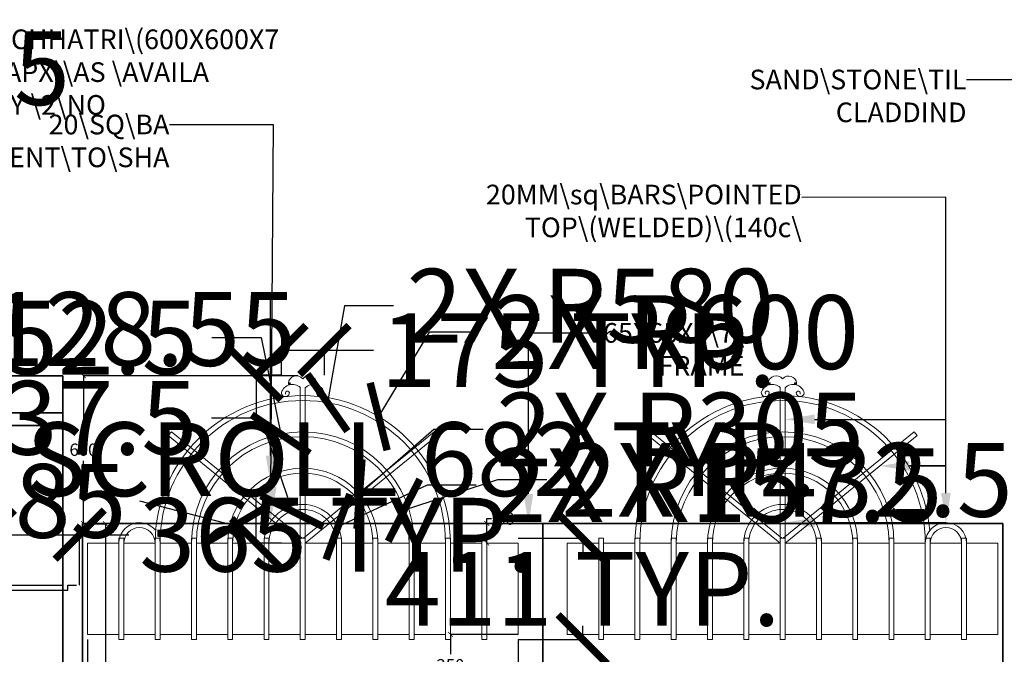
# Model space of a CAD drawing. Units: millimetres. Extents: x 16635 to 28332, y 17519 to 22633.
# Tile 3 of 4: x 20029 to 24031, y 20054 to 22633. Entities that reach past the tile are written whole.
import ezdxf
from ezdxf import colors
from ezdxf.entities.mleader import LeaderData, LeaderLine
from ezdxf.math import Vec2, Vec3

# ---------------------------------------------------------------- set-up
doc = ezdxf.new("R2010")
doc.units = ezdxf.units.MM
doc.header["$MEASUREMENT"] = 0
for name, color, linetype, lineweight in [('A-ANNO-DIMS', 2, 'Continuous', 18), ('A-ANNO-TEXT', 7, 'Continuous', 18), ('A-GATE', 3, 'Continuous', 35), ('A-GATE-GRIL', 4, 'Continuous', 18), ('A-GATE-HRDW', 3, 'Continuous', 25), ('A-WALL', 7, 'Continuous', 35)]:
    doc.layers.add(name, color=color, linetype=linetype, lineweight=lineweight)
doc.styles.get("Standard").update_dxf_attribs({"font": 'arial.ttf'})
doc.dimstyles.get("Standard").update_dxf_attribs({"dimtxt": 300, "dimasz": 200, "dimexe": 0.18, "dimexo": 0.0625, "dimgap": 0.09, "dimtad": 0, "dimtih": 1, "dimtoh": 1, "dimdec": 0, "dimzin": 0, "dimdsep": 46, "dimtxsty": 'Standard', "dimblk": 'ARCHTICK', "dimcen": 0.09, "dimadec": 0, "dimazin": 0, "dimtfac": 1, "dimtdec": 0, "dimtofl": 0, "dimtmove": 0, "dimatfit": 3, "dimfxl": 1, "dimtolj": 1, "dimtzin": 0, "dimarcsym": 0})

# ---------------------------------------------------------------- blocks, each defined once
blk = doc.blocks.new('_ArchTick')
at = {"color": 0, "linetype": 'ByBlock', "const_width": 0.15}
blk.add_lwpolyline([(-0.5, -0.5), (0.5, 0.5)], dxfattribs=at)
blk = doc.blocks.new('*D8')
at = {"layer": 'A-ANNO-DIMS', "color": 0, "lineweight": -2, "transparency": 16777216}
for p, q in [((21159.1, 21185.3), (20288.1, 21185.3)), ((20288.3, 21185.3), (20288.3, 20930.9)), ((20288.3, 20585.3), (20288.3, 20839.8)), ((20284.8, 20585.3), (20288.5, 20585.3))]:
    blk.add_line(p, q, dxfattribs=at)
at = {"layer": 'Defpoints', "color": 0, "transparency": 16777216}
for p in [(20288.3, 21185.3), (21159.1, 21185.3), (20284.8, 20585.3)]:
    blk.add_point(p, dxfattribs=at)
at = {"layer": 'A-ANNO-DIMS', "color": 0, "lineweight": -2, "transparency": 16777216, "xscale": 20, "yscale": 20, "zscale": 20}
for p, rotation in [((20288.3, 21185.3), 90), ((20288.3, 20585.3), 270)]:
    blk.add_blockref('_ArchTick', p, dxfattribs=dict(at, rotation=rotation))
at = {"layer": 'A-ANNO-DIMS', "color": 0, "transparency": 16777216, "insert": (20288.3, 20885.3), "char_height": 50, "attachment_point": 5}
blk.add_mtext('\\A1;600', dxfattribs=at)
blk = doc.blocks.new('*D13')
at = {"layer": 'A-ANNO-DIMS', "color": 0, "lineweight": -2, "transparency": 16777216}
for p, q in [((20284.8, 20584.3), (20377.6, 20584.3)), ((20377.4, 20584.3), (20377.4, 19704.9)), ((20377.4, 18734.3), (20377.4, 19613.8)), ((20284.8, 18734.3), (20377.6, 18734.3))]:
    blk.add_line(p, q, dxfattribs=at)
at = {"layer": 'Defpoints', "color": 0, "transparency": 16777216}
for p in [(20284.8, 20584.3), (20284.8, 18734.3), (20377.4, 18734.3)]:
    blk.add_point(p, dxfattribs=at)
at = {"layer": 'A-ANNO-DIMS', "color": 0, "lineweight": -2, "transparency": 16777216, "xscale": 20, "yscale": 20, "zscale": 20}
for p, rotation in [((20377.4, 20584.3), 90), ((20377.4, 18734.3), 270)]:
    blk.add_blockref('_ArchTick', p, dxfattribs=dict(at, rotation=rotation))
at = {"layer": 'A-ANNO-DIMS', "color": 0, "transparency": 16777216, "insert": (20377.4, 19659.3), "char_height": 50, "attachment_point": 5}
blk.add_mtext('\\A1;1850', dxfattribs=at)
blk = doc.blocks.new('*D14')
at = {"layer": 'A-ANNO-DIMS', "color": 0, "lineweight": -2, "transparency": 16777216}
for p, q in [((22054.7, 20134.3), (21779.6, 20134.3)), ((21779.8, 20134.3), (21779.8, 20054.9)), ((21779.8, 19884.3), (21779.8, 19963.8)), ((22054.7, 19884.3), (21779.6, 19884.3))]:
    blk.add_line(p, q, dxfattribs=at)
at = {"layer": 'Defpoints', "color": 0, "transparency": 16777216}
for p in [(22054.8, 20134.3), (21779.8, 19884.3), (22054.8, 19884.3)]:
    blk.add_point(p, dxfattribs=at)
at = {"layer": 'A-ANNO-DIMS', "color": 0, "lineweight": -2, "transparency": 16777216, "xscale": 20, "yscale": 20, "zscale": 20}
for p, rotation in [((21779.8, 20134.3), 90), ((21779.8, 19884.3), 270)]:
    blk.add_blockref('_ArchTick', p, dxfattribs=dict(at, rotation=rotation))
at = {"layer": 'A-ANNO-DIMS', "color": 0, "transparency": 16777216, "insert": (21779.8, 20009.3), "char_height": 50, "attachment_point": 5}
blk.add_mtext('\\A1;250', dxfattribs=at)
blk = doc.blocks.new('*D15')
at = {"layer": 'A-ANNO-DIMS', "color": 0, "lineweight": -2, "transparency": 16777216}
for p, q in [((21927.3, 20585.3), (21927.3, 20605.3)), ((21927.3, 20605.3), (21947.3, 20605.3)), ((21927.3, 20585.3), (21927.5, 20585.3)), ((21927.3, 20505.3), (21927.3, 20585.3)), ((21927.3, 20505.3), (21927.5, 20505.3))]:
    blk.add_line(p, q, dxfattribs=at)
at = {"layer": 'Defpoints', "color": 0, "transparency": 16777216}
for p in [(21927.3, 20585.3), (21927.3, 20585.3), (21927.3, 20505.3)]:
    blk.add_point(p, dxfattribs=at)
at = {"layer": 'A-ANNO-DIMS', "color": 0, "lineweight": -2, "transparency": 16777216, "xscale": 20, "yscale": 20, "zscale": 20}
for p, rotation in [((21927.3, 20585.3), 90), ((21927.3, 20505.3), 270)]:
    blk.add_blockref('_ArchTick', p, dxfattribs=dict(at, rotation=rotation))
at = {"layer": 'A-ANNO-DIMS', "color": 0, "transparency": 16777216, "insert": (22003, 20605.3), "char_height": 50, "attachment_point": 5}
blk.add_mtext('\\A1;80', dxfattribs=at)
blk = doc.blocks.new('GATE-GRILLE-UPPER')
for p, q in [((127.5, 391), (127.5, 411)), ((127.5, 411), (147.5, 411)), ((147.5, 411), (147.5, 391)), ((275, 391), (275, 411)), ((275, 411), (295, 411)), ((295, 411), (295, 391)), ((422.5, 391), (422.5, 411)), ((422.5, 411), (442.5, 411)), ((442.5, 411), (442.5, 391)), ((570, 391), (570, 411)), ((570, 411), (590, 411)), ((590, 411), (590, 391)), ((717.5, 391), (717.5, 411)), ((717.5, 411), (737.5, 411)), ((737.5, 411), (737.5, 391)), ((865, 411), (885, 411)), ((1012.5, 391), (1012.5, 411)), ((1012.5, 411), (1032.5, 411)), ((1032.5, 411), (1032.5, 391)), ((1160, 391), (1160, 411)), ((1160, 411), (1180, 411)), ((1180, 411), (1180, 391)), ((1307.5, 391), (1307.5, 411)), ((1307.5, 411), (1327.5, 411)), ((1327.5, 411), (1327.5, 391)), ((1455, 391), (1455, 411)), ((1455, 411), (1475, 411)), ((1475, 411), (1475, 391)), ((1602.5, 391), (1602.5, 411)), ((1602.5, 411), (1622.5, 411)), ((1622.5, 411), (1622.5, 391)), ((0, 20), (0, 391)), ((0, 391), (127.5, 391)), ((127.5, 20), (127.5, 391)), ((127.5, 390.5), (127.5, 391)), ((147.5, 20), (147.5, 391)), ((147.5, 390.5), (147.5, 391)), ((147.5, 391), (275, 391)), ((275, 20), (275, 391)), ((275, 390.5), (275, 391)), ((295, 20), (295, 391)), ((295, 390.5), (295, 391)), ((295, 391), (422.5, 391)), ((422.5, 20), (422.5, 391)), ((422.5, 390.5), (422.5, 391)), ((442.5, 20), (442.5, 391)), ((442.5, 390.5), (442.5, 391)), ((442.5, 391), (570, 391)), ((570, 20), (570, 391)), ((570, 390.5), (570, 391)), ((590, 20), (590, 391)), ((590, 390.5), (590, 391)), ((590, 391), (717.5, 391)), ((717.5, 20), (717.5, 391)), ((717.5, 390.5), (717.5, 391)), ((737.5, 20), (737.5, 391)), ((737.5, 390.5), (737.5, 391)), ((737.5, 391), (865, 391)), ((865, 20), (865, 391)), ((865, 390.5), (865, 391)), ((885, 20), (885, 391)), ((885, 390.5), (885, 391)), ((885, 391), (1012.5, 391)), ((1012.5, 20), (1012.5, 391)), ((1012.5, 390.5), (1012.5, 391)), ((1032.5, 20), (1032.5, 391)), ((1032.5, 390.5), (1032.5, 391)), ((1032.5, 391), (1160, 391)), ((1160, 20), (1160, 391)), ((1160, 390.5), (1160, 391)), ((1180, 20), (1180, 391)), ((1180, 390.5), (1180, 391)), ((1180, 391), (1307.5, 391)), ((1307.5, 20), (1307.5, 391)), ((1307.5, 390.5), (1307.5, 391)), ((1327.5, 20), (1327.5, 391)), ((1327.5, 390.5), (1327.5, 391)), ((1327.5, 391), (1455, 391)), ((1455, 20), (1455, 391)), ((1455, 390.5), (1455, 391)), ((1475, 20), (1475, 391)), ((1475, 390.5), (1475, 391)), ((1475, 391), (1602.5, 391)), ((1602.5, 20), (1602.5, 391)), ((1602.5, 390.5), (1602.5, 391)), ((1622.5, 20), (1622.5, 391)), ((1622.5, 390.5), (1622.5, 391)), ((1622.5, 391), (1750, 391)), ((1750, 20), (1750, 391)), ((1750, 390.5), (1750, 391)), ((0, 20), (127.5, 20)), ((127.5, 20), (127.5, 0)), ((147.5, 0), (147.5, 20)), ((147.5, 20), (275, 20)), ((275, 20), (275, 0)), ((295, 0), (295, 20)), ((295, 20), (422.5, 20)), ((422.5, 20), (422.5, 0)), ((442.5, 0), (442.5, 20)), ((442.5, 20), (570, 20)), ((570, 20), (570, 0)), ((590, 0), (590, 20)), ((590, 20), (717.5, 20)), ((717.5, 20), (717.5, 0)), ((737.5, 0), (737.5, 20)), ((737.5, 20), (865, 20)), ((865, 20), (865, 0)), ((885, 0), (885, 20)), ((885, 20), (1012.5, 20)), ((1012.5, 20), (1012.5, 0)), ((1032.5, 0), (1032.5, 20)), ((1032.5, 20), (1160, 20)), ((1160, 20), (1160, 0)), ((1180, 0), (1180, 20)), ((1180, 20), (1307.5, 20)), ((1307.5, 20), (1307.5, 0)), ((1327.5, 0), (1327.5, 20)), ((1327.5, 20), (1455, 20)), ((1455, 20), (1455, 0)), ((1475, 0), (1475, 20)), ((1475, 20), (1602.5, 20)), ((1602.5, 20), (1602.5, 0)), ((1622.5, 0), (1622.5, 20)), ((1622.5, 20), (1750, 20)), ((127.5, 0), (147.5, 0)), ((275, 0), (295, 0)), ((422.5, 0), (442.5, 0)), ((570, 0), (590, 0)), ((717.5, 0), (737.5, 0)), ((865, 0), (885, 0)), ((1012.5, 0), (1032.5, 0)), ((1160, 0), (1180, 0)), ((1307.5, 0), (1327.5, 0)), ((1455, 0), (1475, 0)), ((1602.5, 0), (1622.5, 0))]:
    blk.add_line(p, q)
blk = doc.blocks.new('GATE-CREST-SCROLL')
for p, q in [((76.7, 0), (76.7, 632.5)), ((96.7, 632.1), (96.7, 0))]:
    blk.add_line(p, q)
for centre, radius, start, end in [((44.6, 598.6), 46.7, 46.5386, 162.6285), ((61.2, 646.7), 33.3, 40.0087, 174.5179), ((32.3, 649.8), 4.3, 170.4451, 358.3477), ((34.4, 649.3), 2.21, 12.093, 205.0593), ((111.4, 647.2), 32.3, 5.8157, 139.8182), ((129.3, 598.6), 46.7, 15.1459, 134.1823), ((137.2, 649.2), 2.21, 334.9407, 167.907), ((139.3, 649.8), 4.3, 181.6523, 9.5549), ((16.2, 611.9), 16.2, 177.7213, 358.3477), ((24.2, 609.7), 8.33, 12.093, 205.0593), ((150.2, 609.7), 8.33, 334.9407, 167.907), ((158.2, 611.9), 16.2, 181.6523, 356.1099)]:
    blk.add_arc(centre, radius, start, end)
blk = doc.blocks.new('GATE-JAMB-ANCHOR-SET')
for p, q in [((0.2, 1370), (297.2, 1370)), ((317.2, 1350), (317.2, 1370)), ((317.2, 1370), (351.9, 1370)), ((0.2, 1350), (297.2, 1350)), ((297.2, 1350), (317.2, 1350)), ((0, 694.8), (297, 694.8)), ((317, 674.8), (317, 694.8)), ((317, 694.8), (365.3, 694.8)), ((0, 674.8), (297, 674.8)), ((297, 674.8), (317, 674.8)), ((0.2, 20), (297.2, 20)), ((317.2, 0), (317.2, 20)), ((317.2, 20), (360.9, 20)), ((0.2, 0), (297.2, 0)), ((297.2, 0), (317.2, 0))]:
    blk.add_line(p, q)
blk = doc.blocks.new('*D45')
at = {"layer": 'A-ANNO-DIMS', "color": 0, "lineweight": -2, "transparency": 16777216}
for p, q in [((20304.8, 20114.3), (20304.8, 19851.7)), ((22054.8, 20114.3), (22054.8, 19851.7)), ((20304.8, 19851.8), (22054.8, 19851.8)), ((22054.8, 19851.8), (22254.8, 19851.8))]:
    blk.add_line(p, q, dxfattribs=at)
at = {"layer": 'Defpoints', "color": 0, "transparency": 16777216}
for p in [(20304.8, 20114.3), (22054.8, 20114.3), (22054.8, 19851.8)]:
    blk.add_point(p, dxfattribs=at)
at = {"layer": 'A-ANNO-DIMS', "color": 0, "lineweight": -2, "transparency": 16777216, "xscale": 200, "yscale": 200, "zscale": 200, "rotation": 180}
blk.add_blockref('_ArchTick', (20304.8, 19851.8), dxfattribs=at)
at = {"layer": 'A-ANNO-DIMS', "color": 0, "lineweight": -2, "transparency": 16777216, "xscale": 200, "yscale": 200, "zscale": 200}
blk.add_blockref('_ArchTick', (22054.8, 19851.8), dxfattribs=at)
at = {"layer": 'A-ANNO-DIMS', "color": 0, "transparency": 16777216, "insert": (24794.1, 19851.8), "char_height": 300, "attachment_point": 5}
blk.add_mtext('\\A1;UPPER GRILLE 1750 TYP.', dxfattribs=at)
blk = doc.blocks.new('*D46')
at = {"layer": 'A-ANNO-DIMS', "color": 0, "lineweight": -2, "transparency": 16777216}
for p, q in [((22054.8, 20525.3), (22317.5, 20525.3)), ((22317.3, 20525.3), (22317.3, 20470.7)), ((22317.3, 20114.3), (22317.3, 20169)), ((22054.8, 20114.3), (22317.5, 20114.3))]:
    blk.add_line(p, q, dxfattribs=at)
at = {"layer": 'Defpoints', "color": 0, "transparency": 16777216}
for p in [(22054.8, 20525.3), (22317.3, 20525.3), (22054.8, 20114.3)]:
    blk.add_point(p, dxfattribs=at)
at = {"layer": 'A-ANNO-DIMS', "color": 0, "lineweight": -2, "transparency": 16777216, "xscale": 200, "yscale": 200, "zscale": 200}
for p, rotation in [((22317.3, 20525.3), 90), ((22317.3, 20114.3), 270)]:
    blk.add_blockref('_ArchTick', p, dxfattribs=dict(at, rotation=rotation))
at = {"layer": 'A-ANNO-DIMS', "color": 0, "transparency": 16777216, "insert": (22317.3, 20319.8), "char_height": 300, "attachment_point": 5}
blk.add_mtext('\\A1;411 TYP.', dxfattribs=at)
blk = doc.blocks.new('*D47')
at = {"layer": 'A-ANNO-DIMS', "color": 0, "lineweight": -2, "transparency": 16777216}
for p, q in [((21092.8, 21187.8), (20990.3, 21187.8)), ((20990.5, 21187.8), (20990.5, 21001.9)), ((20990.5, 20505.3), (20990.5, 20691.3)), ((21092.8, 20505.3), (20990.3, 20505.3))]:
    blk.add_line(p, q, dxfattribs=at)
at = {"layer": 'Defpoints', "color": 0, "transparency": 16777216}
for p in [(20990.5, 21187.8), (21092.8, 21187.8), (21092.8, 20505.3)]:
    blk.add_point(p, dxfattribs=at)
at = {"layer": 'A-ANNO-DIMS', "color": 0, "lineweight": -2, "transparency": 16777216, "xscale": 200, "yscale": 200, "zscale": 200}
for p, rotation in [((20990.5, 21187.8), 90), ((20990.5, 20505.3), 270)]:
    blk.add_blockref('_ArchTick', p, dxfattribs=dict(at, rotation=rotation))
at = {"layer": 'A-ANNO-DIMS', "color": 0, "transparency": 16777216, "insert": (20990.5, 20846.6), "char_height": 300, "attachment_point": 5}
blk.add_mtext('\\A1;CREST SCROLL 682 TYP.', dxfattribs=at)
blk = doc.blocks.new('*D48')
at = {"layer": 'A-ANNO-DIMS', "color": 0, "lineweight": -2, "transparency": 16777216}
for p, q in [((21092.8, 21187.9), (21092.8, 21290.4)), ((21092.8, 21290.2), (21267.4, 21290.2)), ((21267.4, 21187.9), (21267.4, 21290.4)), ((21267.4, 21290.2), (21467.4, 21290.2))]:
    blk.add_line(p, q, dxfattribs=at)
at = {"layer": 'Defpoints', "color": 0, "transparency": 16777216}
for p in [(21267.4, 21290.2), (21092.8, 21187.8), (21267.4, 21187.8)]:
    blk.add_point(p, dxfattribs=at)
at = {"layer": 'A-ANNO-DIMS', "color": 0, "lineweight": -2, "transparency": 16777216, "xscale": 200, "yscale": 200, "zscale": 200, "rotation": 180}
blk.add_blockref('_ArchTick', (21092.8, 21290.2), dxfattribs=at)
at = {"layer": 'A-ANNO-DIMS', "color": 0, "lineweight": -2, "transparency": 16777216, "xscale": 200, "yscale": 200, "zscale": 200}
blk.add_blockref('_ArchTick', (21267.4, 21290.2), dxfattribs=at)
at = {"layer": 'A-ANNO-DIMS', "color": 0, "transparency": 16777216, "insert": (22300.1, 21290.2), "char_height": 300, "attachment_point": 5}
blk.add_mtext('\\A1;175 TYP.', dxfattribs=at)
blk = doc.blocks.new('*D49')
at = {"layer": 'A-ANNO-DIMS', "color": 0, "lineweight": -2, "transparency": 16777216}
for p, q in [((19907.5, 20334.3), (19701.9, 20334.3)), ((19702.1, 20334.3), (19702.1, 19804.8)), ((19702.1, 18964.3), (19702.1, 19493.9)), ((19907.5, 18964.3), (19701.9, 18964.3))]:
    blk.add_line(p, q, dxfattribs=at)
at = {"layer": 'Defpoints', "color": 0, "transparency": 16777216}
for p in [(19702.1, 20334.3), (19907.6, 20334.3), (19907.6, 18964.3)]:
    blk.add_point(p, dxfattribs=at)
at = {"layer": 'A-ANNO-DIMS', "color": 0, "lineweight": -2, "transparency": 16777216, "xscale": 200, "yscale": 200, "zscale": 200}
for p, rotation in [((19702.1, 20334.3), 90), ((19702.1, 18964.3), 270)]:
    blk.add_blockref('_ArchTick', p, dxfattribs=dict(at, rotation=rotation))
at = {"layer": 'A-ANNO-DIMS', "color": 0, "transparency": 16777216, "insert": (19702.1, 19649.3), "char_height": 300, "attachment_point": 5}
blk.add_mtext('\\A1;JAMB ANCHORS 1370 TYP.', dxfattribs=at)
blk = doc.blocks.new('*D50')
at = {"layer": 'A-ANNO-DIMS', "color": 0, "lineweight": -2, "transparency": 16777216}
for p, q in [((19907.6, 20334.4), (19907.6, 20540)), ((19907.6, 20539.8), (20272.8, 20539.8)), ((20272.8, 20334.4), (20272.8, 20540)), ((20272.8, 20539.8), (20472.8, 20539.8))]:
    blk.add_line(p, q, dxfattribs=at)
at = {"layer": 'Defpoints', "color": 0, "transparency": 16777216}
for p in [(20272.8, 20539.8), (19907.6, 20334.3), (20272.8, 20334.3)]:
    blk.add_point(p, dxfattribs=at)
at = {"layer": 'A-ANNO-DIMS', "color": 0, "lineweight": -2, "transparency": 16777216, "xscale": 200, "yscale": 200, "zscale": 200, "rotation": 180}
blk.add_blockref('_ArchTick', (19907.6, 20539.8), dxfattribs=at)
at = {"layer": 'A-ANNO-DIMS', "color": 0, "lineweight": -2, "transparency": 16777216, "xscale": 200, "yscale": 200, "zscale": 200}
blk.add_blockref('_ArchTick', (20272.8, 20539.8), dxfattribs=at)
at = {"layer": 'A-ANNO-DIMS', "color": 0, "transparency": 16777216, "insert": (21319.5, 20539.8), "char_height": 300, "attachment_point": 5}
blk.add_mtext('\\A1;365 TYP.', dxfattribs=at)
blk = doc.blocks.new('*D59')
at = {"layer": 'A-ANNO-DIMS', "color": 0, "lineweight": -2, "transparency": 16777216}
for p, q in [((18754.8, 20334.4), (18754.8, 22436.4)), ((18754.8, 22436.2), (19012.3, 22436.2)), ((19012.3, 21184.4), (19012.3, 22436.4)), ((19012.3, 22436.2), (19212.3, 22436.2))]:
    blk.add_line(p, q, dxfattribs=at)
at = {"layer": 'Defpoints', "color": 0, "transparency": 16777216}
for p in [(19012.3, 22436.2), (19012.3, 21184.3), (18754.8, 20334.3)]:
    blk.add_point(p, dxfattribs=at)
at = {"layer": 'A-ANNO-DIMS', "color": 0, "lineweight": -2, "transparency": 16777216, "xscale": 200, "yscale": 200, "zscale": 200, "rotation": 180}
blk.add_blockref('_ArchTick', (18754.8, 22436.2), dxfattribs=at)
at = {"layer": 'A-ANNO-DIMS', "color": 0, "lineweight": -2, "transparency": 16777216, "xscale": 200, "yscale": 200, "zscale": 200}
blk.add_blockref('_ArchTick', (19012.3, 22436.2), dxfattribs=at)
at = {"layer": 'A-ANNO-DIMS', "color": 0, "transparency": 16777216, "insert": (19722.2, 22436.2), "char_height": 300, "attachment_point": 5}
blk.add_mtext('\\A1;257.5', dxfattribs=at)
blk = doc.blocks.new('*D66')
at = {"layer": 'A-ANNO-DIMS', "color": 0, "lineweight": -2, "transparency": 16777216}
for p, q in [((19003.3, 21688.7), (19003.5, 21688.7)), ((19003.4, 21688.6), (19003.4, 21688.7)), ((19429.5, 21375.9), (19107.1, 21612.6)), ((19629.5, 21375.9), (19429.5, 21375.9))]:
    blk.add_line(p, q, dxfattribs=at)
at = {"layer": 'Defpoints', "color": 0, "transparency": 16777216}
for p in [(19003.4, 21688.7), (19107.1, 21612.6)]:
    blk.add_point(p, dxfattribs=at)
at = {"layer": 'A-ANNO-DIMS', "color": 0, "lineweight": -2, "transparency": 16777216, "xscale": 200, "yscale": 200, "zscale": 200, "rotation": 143.726603085954}
blk.add_blockref('_ArchTick', (19107.1, 21612.6), dxfattribs=at)
at = {"layer": 'A-ANNO-DIMS', "color": 0, "transparency": 16777216, "insert": (20397, 21375.9), "char_height": 300, "attachment_point": 5}
blk.add_mtext('\\A1;R128.55', dxfattribs=at)
blk = doc.blocks.new('*D67')
at = {"layer": 'A-ANNO-DIMS', "color": 0, "lineweight": -2, "transparency": 16777216}
for p, q in [((21693.6, 21363.3), (21488.1, 21020.1)), ((21893.6, 21363.3), (21693.6, 21363.3)), ((21179.7, 20505.3), (21179.9, 20505.3)), ((21179.8, 20505.3), (21179.8, 20505.4))]:
    blk.add_line(p, q, dxfattribs=at)
at = {"layer": 'Defpoints', "color": 0, "transparency": 16777216}
for p in [(21488.1, 21020.1), (21179.8, 20505.3)]:
    blk.add_point(p, dxfattribs=at)
at = {"layer": 'A-ANNO-DIMS', "color": 0, "lineweight": -2, "transparency": 16777216, "xscale": 200, "yscale": 200, "zscale": 200, "rotation": 239.0822028428942}
blk.add_blockref('_ArchTick', (21488.1, 21020.1), dxfattribs=at)
at = {"layer": 'A-ANNO-DIMS', "color": 0, "transparency": 16777216, "insert": (22693, 21363.3), "char_height": 300, "attachment_point": 5}
blk.add_mtext('\\A1;2X R600', dxfattribs=at)
blk = doc.blocks.new('*D68')
at = {"layer": 'A-ANNO-DIMS', "color": 0, "lineweight": -2, "transparency": 16777216}
for p, q in [((21349, 21470.6), (21279.9, 21076.6)), ((21549, 21470.6), (21349, 21470.6)), ((21179.7, 20505.3), (21179.9, 20505.3)), ((21179.8, 20505.3), (21179.8, 20505.4))]:
    blk.add_line(p, q, dxfattribs=at)
at = {"layer": 'Defpoints', "color": 0, "transparency": 16777216}
for p in [(21279.9, 21076.6), (21179.8, 20505.3)]:
    blk.add_point(p, dxfattribs=at)
at = {"layer": 'A-ANNO-DIMS', "color": 0, "lineweight": -2, "transparency": 16777216, "xscale": 200, "yscale": 200, "zscale": 200, "rotation": 260.0552103335245}
blk.add_blockref('_ArchTick', (21279.9, 21076.6), dxfattribs=at)
at = {"layer": 'A-ANNO-DIMS', "color": 0, "transparency": 16777216, "insert": (22348.4, 21470.6), "char_height": 300, "attachment_point": 5}
blk.add_mtext('\\A1;2X R580', dxfattribs=at)
blk = doc.blocks.new('*D69')
at = {"layer": 'A-ANNO-DIMS', "color": 0, "lineweight": -2, "transparency": 16777216}
for p, q in [((20810.7, 21340.9), (21010.7, 21340.9)), ((21010.7, 21340.9), (21090, 20948.9)), ((21179.7, 20505.3), (21179.9, 20505.3)), ((21179.8, 20505.3), (21179.8, 20505.4))]:
    blk.add_line(p, q, dxfattribs=at)
at = {"layer": 'Defpoints', "color": 0, "transparency": 16777216}
for p in [(21090, 20948.9), (21179.8, 20505.3)]:
    blk.add_point(p, dxfattribs=at)
at = {"layer": 'A-ANNO-DIMS', "color": 0, "lineweight": -2, "transparency": 16777216, "xscale": 200, "yscale": 200, "zscale": 200, "rotation": 281.4390211623567}
blk.add_blockref('_ArchTick', (21090, 20948.9), dxfattribs=at)
at = {"layer": 'A-ANNO-DIMS', "color": 0, "transparency": 16777216, "insert": (19834.9, 21340.9), "char_height": 300, "attachment_point": 5}
blk.add_mtext('\\A1;2X R452.5', dxfattribs=at)
blk = doc.blocks.new('*D70')
at = {"layer": 'A-ANNO-DIMS', "color": 0, "lineweight": -2, "transparency": 16777216}
for p, q in [((21971.5, 20762.6), (21591.1, 20639)), ((22171.5, 20762.6), (21971.5, 20762.6)), ((21179.7, 20505.3), (21179.9, 20505.3)), ((21179.8, 20505.3), (21179.8, 20505.4))]:
    blk.add_line(p, q, dxfattribs=at)
at = {"layer": 'Defpoints', "color": 0, "transparency": 16777216}
for p in [(21591.1, 20639), (21179.8, 20505.3)]:
    blk.add_point(p, dxfattribs=at)
at = {"layer": 'A-ANNO-DIMS', "color": 0, "lineweight": -2, "transparency": 16777216, "xscale": 200, "yscale": 200, "zscale": 200, "rotation": 198.0002935108227}
blk.add_blockref('_ArchTick', (21591.1, 20639), dxfattribs=at)
at = {"layer": 'A-ANNO-DIMS', "color": 0, "transparency": 16777216, "insert": (23147.3, 20762.6), "char_height": 300, "attachment_point": 5}
blk.add_mtext('\\A1;2X R432.5', dxfattribs=at)
blk = doc.blocks.new('*D71')
at = {"layer": 'A-ANNO-DIMS', "color": 0, "lineweight": -2, "transparency": 16777216}
for p, q in [((21712.4, 20967.2), (21410.2, 20705.2)), ((21912.4, 20967.2), (21712.4, 20967.2)), ((21179.7, 20505.3), (21179.9, 20505.3)), ((21179.8, 20505.3), (21179.8, 20505.4))]:
    blk.add_line(p, q, dxfattribs=at)
at = {"layer": 'Defpoints', "color": 0, "transparency": 16777216}
for p in [(21410.2, 20705.2), (21179.8, 20505.3)]:
    blk.add_point(p, dxfattribs=at)
at = {"layer": 'A-ANNO-DIMS', "color": 0, "lineweight": -2, "transparency": 16777216, "xscale": 200, "yscale": 200, "zscale": 200, "rotation": 220.9312972223516}
blk.add_blockref('_ArchTick', (21410.2, 20705.2), dxfattribs=at)
at = {"layer": 'A-ANNO-DIMS', "color": 0, "transparency": 16777216, "insert": (22713.4, 20967.2), "char_height": 300, "attachment_point": 5}
blk.add_mtext('\\A1;2X R305', dxfattribs=at)
blk = doc.blocks.new('*D72')
at = {"layer": 'A-ANNO-DIMS', "color": 0, "lineweight": -2, "transparency": 16777216}
for p, q in [((20516.7, 20677.3), (20903.9, 20576.9)), ((21179.7, 20505.3), (21179.9, 20505.3)), ((21179.8, 20505.3), (21179.8, 20505.4))]:
    blk.add_line(p, q, dxfattribs=at)
at = {"layer": 'Defpoints', "color": 0, "transparency": 16777216}
for p in [(20903.9, 20576.9), (21179.8, 20505.3)]:
    blk.add_point(p, dxfattribs=at)
at = {"layer": 'A-ANNO-DIMS', "color": 0, "lineweight": -2, "transparency": 16777216, "xscale": 200, "yscale": 200, "zscale": 200, "rotation": 345.4648454983082}
blk.add_blockref('_ArchTick', (20903.9, 20576.9), dxfattribs=at)
at = {"layer": 'A-ANNO-DIMS', "color": 0, "transparency": 16777216, "insert": (19715.6, 20677.3), "char_height": 300, "attachment_point": 5}
blk.add_mtext('\\A1;2X R285', dxfattribs=at)
blk = doc.blocks.new('*D73')
at = {"layer": 'A-ANNO-DIMS', "color": 0, "lineweight": -2, "transparency": 16777216}
for p, q in [((21685, 20740.9), (21322.5, 20571.9)), ((21885, 20740.9), (21685, 20740.9)), ((21179.7, 20505.3), (21179.9, 20505.3)), ((21179.8, 20505.3), (21179.8, 20505.4))]:
    blk.add_line(p, q, dxfattribs=at)
at = {"layer": 'Defpoints', "color": 0, "transparency": 16777216}
for p in [(21322.5, 20571.9), (21179.8, 20505.3)]:
    blk.add_point(p, dxfattribs=at)
at = {"layer": 'A-ANNO-DIMS', "color": 0, "lineweight": -2, "transparency": 16777216, "xscale": 200, "yscale": 200, "zscale": 200, "rotation": 204.9969783898798}
blk.add_blockref('_ArchTick', (21322.5, 20571.9), dxfattribs=at)
at = {"layer": 'A-ANNO-DIMS', "color": 0, "transparency": 16777216, "insert": (22860.9, 20740.9), "char_height": 300, "attachment_point": 5}
blk.add_mtext('\\A1;2X R157.5', dxfattribs=at)
blk = doc.blocks.new('*D74')
at = {"layer": 'A-ANNO-DIMS', "color": 0, "lineweight": -2, "transparency": 16777216}
for p, q in [((20809, 21015), (21009, 21015)), ((21009, 21015), (21136.1, 20635.7)), ((21179.7, 20505.3), (21179.9, 20505.3)), ((21179.8, 20505.3), (21179.8, 20505.4))]:
    blk.add_line(p, q, dxfattribs=at)
at = {"layer": 'Defpoints', "color": 0, "transparency": 16777216}
for p in [(21136.1, 20635.7), (21179.8, 20505.3)]:
    blk.add_point(p, dxfattribs=at)
at = {"layer": 'A-ANNO-DIMS', "color": 0, "lineweight": -2, "transparency": 16777216, "xscale": 200, "yscale": 200, "zscale": 200, "rotation": 288.5216632841473}
blk.add_blockref('_ArchTick', (21136.1, 20635.7), dxfattribs=at)
at = {"layer": 'A-ANNO-DIMS', "color": 0, "transparency": 16777216, "insert": (19833.2, 21015), "char_height": 300, "attachment_point": 5}
blk.add_mtext('\\A1;2X R137.5', dxfattribs=at)

msp = doc.modelspace()

# ---------------------------------------------------------------- linework, layer by layer
at = {"layer": 'A-GATE'}
for p, q in [((20284.77, 18734.349), (20284.77, 20585.349)), ((20284.77, 20585.349), (22074.77, 20585.349)), ((22074.77, 20585.349), (24024.77, 20585.349)), ((22154.77, 18734.349), (22154.77, 20585.349)), ((24024.77, 18734.349), (24024.77, 20585.349))]:
    msp.add_line(p, q, dxfattribs=at)
at = {"layer": 'A-GATE-GRIL'}
for p, q in [((20645.782, 20957.959), (20633.069, 20942.519)), ((20633.069, 20942.519), (21169.77, 20505.349)), ((21176.885, 20525.349), (20645.782, 20957.959)), ((21182.656, 20525.349), (21713.759, 20957.959)), ((21726.472, 20942.519), (21189.77, 20505.349)), ((21713.759, 20957.959), (21726.39, 20942.452)), ((22595.782, 20957.959), (22583.069, 20942.519)), ((22583.069, 20942.519), (23119.77, 20505.349)), ((23126.885, 20525.349), (22595.782, 20957.959)), ((23132.656, 20525.349), (23663.759, 20957.959)), ((23676.472, 20942.519), (23139.77, 20505.349)), ((23663.759, 20957.959), (23676.472, 20942.519)), ((23119.77, 20525.349), (23119.77, 20505.349)), ((23139.77, 20505.349), (23139.77, 20525.349))]:
    msp.add_line(p, q, dxfattribs=at)
for centre, radius, start, end in [((21179.77, 20505.349), 600, 0, 180), ((23129.77, 20505.349), 600, 4.932759, 180), ((21179.77, 20505.349), 580, 0, 180), ((23129.77, 20505.349), 580, 0, 180), ((21179.77, 20505.349), 452.5, 0, 180), ((21179.77, 20505.349), 432.5, 0, 180), ((23129.77, 20505.349), 452.5, 0, 180), ((23129.77, 20505.349), 432.5, 0, 180), ((21179.77, 20505.349), 305, 0, 180), ((23129.77, 20505.349), 305, 0, 180), ((21179.77, 20505.349), 285, 0, 180), ((23129.77, 20505.349), 285, 0, 180), ((21179.77, 20505.349), 157.5, 0, 180), ((23129.77, 20505.349), 157.5, 0, 180), ((21179.77, 20505.349), 137.5, 0, 180), ((23129.77, 20505.349), 137.5, 0, 180), ((20516.02, 20505.349), 83.75, 38.026304, 180), ((20516.02, 20505.349), 63.75, 0, 180), ((23793.52, 20505.349), 83.75, 0, 180), ((23793.52, 20505.349), 63.75, 0, 180), ((20516.02, 20505.349), 83.75, 0, 13.816078), ((23129.77, 20505.349), 600, 0, 1.910213)]:
    msp.add_arc(centre, radius, start, end, dxfattribs=at)
at = {"layer": 'A-WALL'}
for p, q in [((20204.77, 21185.349), (18204.77, 21185.349)), ((20204.77, 18584.349), (20204.77, 21185.349)), ((20204.77, 21035.349), (18204.77, 21035.349)), ((20204.77, 20984.349), (18204.77, 20984.349))]:
    msp.add_line(p, q, dxfattribs=at)

# ---------------------------------------------------------------- block references
at = {"layer": 'A-GATE-GRIL'}
for name, p in [('GATE-CREST-SCROLL', (21093.07, 20505.349)), ('GATE-CREST-SCROLL', (23043.07, 20505.349)), ('GATE-GRILLE-UPPER', (20304.77, 20114.349))]:
    msp.add_blockref(name, p, dxfattribs=at)
at = {"layer": 'A-GATE-GRIL', "extrusion": (0, 0, -1), "zscale": -1}
msp.add_blockref('GATE-GRILLE-UPPER', (-24004.771, 20114.349), dxfattribs=at)
at = {"layer": 'A-GATE-HRDW'}
msp.add_blockref('GATE-JAMB-ANCHOR-SET', (19907.57, 18964.349), dxfattribs=at)

# ---------------------------------------------------------------- dimensions: what is measured, and where the dimension line sits
at = {"layer": 'A-ANNO-DIMS'}
dim = msp.add_linear_dim(base=(19012.27, 22436.24), p1=(18754.77, 20334.349), p2=(19012.27, 21184.349), dimstyle='Standard', override={"dimdec": 1, "dimlfac": 1, "dimrnd": 0, "dimzin": 0, "dimdsep": 46, "dimlunit": 2}, dxfattribs=at)
dim.commit()
dim.dimension.update_dxf_attribs({"geometry": '*D59', "text_midpoint": (19722.217, 22436.24)})
for mpoint, override, picture, middle in [((21279.936, 21076.634), {"dimdec": 0, "dimlfac": 1, "dimrnd": 0, "dimzin": 0, "dimdsep": 46, "dimlunit": 2}, '*D68', (22348.423, 21470.624)), ((21488.055, 21020.092), {"dimdec": 0, "dimlfac": 1, "dimrnd": 0, "dimzin": 0, "dimdsep": 46, "dimlunit": 2}, '*D67', (22692.986, 21363.254)), ((21090.028, 20948.86), {"dimdec": 1, "dimlfac": 1, "dimrnd": 0, "dimzin": 0, "dimdsep": 46, "dimlunit": 2}, '*D69', (19834.892, 21340.915)), ((21136.092, 20635.727), {"dimdec": 1, "dimlfac": 1, "dimrnd": 0, "dimzin": 0, "dimdsep": 46, "dimlunit": 2}, '*D74', (19833.22, 21015.008)), ((21410.196, 20705.17), {"dimdec": 0, "dimlfac": 1, "dimrnd": 0, "dimzin": 0, "dimdsep": 46, "dimlunit": 2}, '*D71', (22713.44, 20967.232)), ((21591.102, 20639.001), {"dimdec": 1, "dimlfac": 1, "dimrnd": 0, "dimzin": 0, "dimdsep": 46, "dimlunit": 2}, '*D70', (23147.33, 20762.609)), ((21322.517, 20571.903), {"dimdec": 1, "dimlfac": 1, "dimrnd": 0, "dimzin": 0, "dimdsep": 46, "dimlunit": 2}, '*D73', (22860.856, 20740.932)), ((20903.892, 20576.876), {"dimdec": 0, "dimlfac": 1, "dimrnd": 0, "dimzin": 0, "dimdsep": 46, "dimlunit": 2}, '*D72', (19715.65, 20677.266))]:
    dim = msp.add_radius_dim(center=(21179.77, 20505.349), mpoint=mpoint, text='2X <>', dimstyle='Standard', override=override, dxfattribs=at)
    dim.commit()
    dim.dimension.update_dxf_attribs({"geometry": picture, "text_midpoint": middle})
for base, p1, p2, text, picture, middle in [((20990.466, 21187.833), (21092.839, 20505.349), (21092.839, 21187.833), 'CREST SCROLL <> TYP.', '*D47', (20990.466, 20846.591)), ((22317.27, 20525.349), (22054.77, 20114.349), (22054.77, 20525.349), '<> TYP.', '*D46', (22317.27, 20319.849)), ((19702.07, 20334.349), (19907.57, 18964.349), (19907.57, 20334.349), 'JAMB ANCHORS <> TYP.', '*D49', (19702.07, 19649.349))]:
    dim = msp.add_linear_dim(base=base, p1=p1, p2=p2, angle=90, text=text, dimstyle='Standard', override={"dimdec": 0, "dimlfac": 1, "dimrnd": 0, "dimzin": 0, "dimdsep": 46, "dimlunit": 2}, dxfattribs=at)
    dim.commit()
    dim.dimension.update_dxf_attribs({"geometry": picture, "text_midpoint": middle})
for base, p1, p2, text, picture, middle in [((21267.403, 21290.206), (21092.839, 21187.833), (21267.403, 21187.833), '<> TYP.', '*D48', (22300.065, 21290.206)), ((20272.849, 20539.849), (19907.57, 20334.349), (20272.849, 20334.349), '<> TYP.', '*D50', (21319.528, 20539.849)), ((22054.77, 19851.849), (20304.77, 20114.349), (22054.77, 20114.349), 'UPPER GRILLE <> TYP.', '*D45', (24794.117, 19851.849))]:
    dim = msp.add_linear_dim(base=base, p1=p1, p2=p2, text=text, dimstyle='Standard', override={"dimdec": 0, "dimlfac": 1, "dimrnd": 0, "dimzin": 0, "dimdsep": 46, "dimlunit": 2}, dxfattribs=at)
    dim.commit()
    dim.dimension.update_dxf_attribs({"geometry": picture, "text_midpoint": middle})
dim = msp.add_radius_dim(center=(19003.421, 21688.654), mpoint=(19107.056, 21612.6), dimstyle='Standard', override={"dimdec": 2, "dimlfac": 1, "dimrnd": 0, "dimzin": 0, "dimdsep": 46, "dimlunit": 2}, dxfattribs=at)
dim.commit()
dim.dimension.update_dxf_attribs({"geometry": '*D66', "text_midpoint": (20397.021, 21375.945)})
for base, p1, p2, picture, middle in [((20288.297, 21185.349), (20284.77, 20585.349), (21159.137, 21185.349), '*D8', (20288.297, 20885.349)), ((21927.27, 20585.349), (21927.27, 20505.349), (21927.27, 20585.349), '*D15', (22003.031, 20605.349)), ((21779.77, 19884.349), (22054.77, 20134.349), (22054.77, 19884.349), '*D14', (21779.77, 20009.349))]:
    dim = msp.add_linear_dim(base=base, p1=p1, p2=p2, angle=90, dimstyle='Standard', override={"dimtxt": 50, "dimasz": 20, "dimgap": 20, "dimclrd": 0, "dimclre": 0, "dimclrt": 0}, dxfattribs=at)
    dim.commit()
    dim.dimension.update_dxf_attribs({"geometry": picture, "text_midpoint": middle})
dim = msp.add_linear_dim(base=(20377.407, 18734.349), p1=(20284.77, 20584.349), p2=(20284.77, 18734.349), angle=90, dimstyle='Standard', override={"dimtxt": 50, "dimasz": 20, "dimgap": 20, "dimclrd": 0, "dimclre": 0, "dimclrt": 0}, dxfattribs=at)
dim.commit()
dim.dimension.update_dxf_attribs({"geometry": '*D13', "text_midpoint": (20377.407, 19659.349), "dimtype": 160})

# ---------------------------------------------------------------- leaders
at = {"layer": 'A-ANNO-TEXT'}
ml = msp.add_multileader_mtext('Standard', dxfattribs=at)
ml.set_content('STONE\\\\CHHATRI\\\\(600X600X7\\PHEIGH\\\\APX)\\\\AS \\\\AVAILA\\PLOCALLY \\\\2\\\\NO', color=256)
ml.set_leader_properties()
ml.build(insert=Vec2(0, 0))
ml.multileader.update_dxf_attribs({"dogleg_length": 0.36, "arrow_head_size": 120})
ctx = ml.context
ctx.base_point, ctx.char_height, ctx.arrow_head_size, ctx.landing_gap_size, ctx.plane_origin = Vec3(19596.252, 22552.693), 80, 120, 0.09, Vec3(18752.322, 23724.498)
notes = []
notes.append((ctx, [(1, (1, 1, 0), (19595.802, 22552.693), (1, 0), 0.45, [(0, [(19337.724, 21745.603), (19337.724, 22543.26)], 0, [])])]))
ctx.mtext.insert, ctx.mtext.flow_direction = Vec3(19596.342, 22593.375), 5
ml = msp.add_multileader_mtext('Standard', dxfattribs=at)
ml.set_content('SAND\\\\STONE\\\\TIL\\PCLADDIND', color=256)
ml.set_leader_properties()
ml.build(insert=Vec2(0, 0))
ml.multileader.update_dxf_attribs({"dogleg_length": 0.36, "arrow_head_size": 120})
ctx = ml.context
ctx.base_point, ctx.char_height, ctx.arrow_head_size, ctx.landing_gap_size, ctx.plane_origin = Vec3(22967.113, 22389.231), 80, 120, 0.09, Vec3(23877.721, 22389.231)
ctx.text_align_type = 2
notes.append((ctx, [(0, (1, 1, 0), (23877.721, 22389.231), (-1, 0), 0.36, [(0, [(24689.11, 19800.774), (24689.11, 22389.231)], 0, [])])]))
ctx.mtext.insert, ctx.mtext.alignment, ctx.mtext.flow_direction = Vec3(23877.271, 22429.914), 3, 5
ml = msp.add_multileader_mtext('Standard', dxfattribs=at)
ml.set_content('20\\\\SQ\\\\BA\\PBENT\\\\TO\\\\SHA', color=256)
ml.set_leader_properties()
ml.build(insert=Vec2(0, 0))
ml.multileader.update_dxf_attribs({"dogleg_length": 0.36, "arrow_head_size": 140})
ctx = ml.context
ctx.base_point, ctx.char_height, ctx.arrow_head_size, ctx.landing_gap_size, ctx.plane_origin = Vec3(19900.508, 22206.331), 80, 140, 0.09, Vec3(20734.191, 21659.695)
ctx.text_align_type = 2
notes.append((ctx, [(0, (1, 1, 0), (20638.183, 22206.331), (-1, 0), 0.36, [(0, [(21049.17, 20593.381), (21060.96, 22205.47)], 0, [])])]))
ctx.mtext.insert, ctx.mtext.alignment, ctx.mtext.flow_direction = Vec3(20637.733, 22247.013), 3, 5
ml = msp.add_multileader_mtext('Standard', dxfattribs=at)
ml.set_content('20MM\\\\sq\\\\BARS\\\\POINTED\\PTOP\\\\(WELDED)\\\\(140c\\\\', color=256)
ml.set_leader_properties()
ml.build(insert=Vec2(0, 0))
ml.multileader.update_dxf_attribs({"dogleg_length": 0.36, "arrow_head_size": 120})
ctx = ml.context
ctx.base_point, ctx.char_height, ctx.arrow_head_size, ctx.landing_gap_size, ctx.plane_origin = Vec3(21894.017, 21910.654), 80, 120, 0.09, Vec3(23208.118, 22419.808)
ctx.text_align_type = 2
notes.append((ctx, [(0, (1, 1, 0), (23208.118, 21910.654), (-1, 0), 0.36, [(0, [(23793.52, 20589.099), (23793.52, 21911.642)], 0, [])])]))
ctx.mtext.insert, ctx.mtext.alignment, ctx.mtext.flow_direction = Vec3(23207.668, 21962.414), 3, 5
ml = msp.add_multileader_mtext('Standard', dxfattribs=at)
ml.set_content('', color=256)
ml.set_leader_properties()
ml.build(insert=Vec2(0, 0))
ml.multileader.update_dxf_attribs({"dogleg_length": 0.36, "arrow_head_size": 120})
ctx = ml.context
ctx.base_point, ctx.char_height, ctx.arrow_head_size, ctx.landing_gap_size, ctx.plane_origin, ctx.plane_x_axis, ctx.plane_y_axis = Vec3(21049.17, 21520.352), 80, 120, 0.09, Vec3(21049.17, 21381.265), Vec3(0, -1), Vec3(1, 0)
ctx.text_align_type = 2
notes.append((ctx, [(0, (1, 1, 0), (21049.17, 21381.265), (0, 1), 138.907, [(0, [(21049.17, 20866.422), (21049.17, 21169.404)], 0, [])])]))
ctx.mtext.insert, ctx.mtext.text_direction, ctx.mtext.rotation, ctx.mtext.alignment, ctx.mtext.flow_direction = Vec3(21089.17, 21520.262), Vec3(0, -1), 4.71238898, 3, 5
ml = msp.add_multileader_mtext('Standard', dxfattribs=at)
ml.set_content('', color=256)
ml.set_leader_properties()
ml.build(insert=Vec2(0, 0))
ml.multileader.update_dxf_attribs({"dogleg_length": 0.36, "arrow_head_size": 120})
ctx = ml.context
ctx.base_point, ctx.char_height, ctx.arrow_head_size, ctx.landing_gap_size, ctx.plane_origin, ctx.plane_x_axis, ctx.plane_y_axis = Vec3(21049.17, 21395.184), 80, 120, 0.09, Vec3(21049.17, 21256.097), Vec3(0, -1), Vec3(1, 0)
ctx.text_align_type = 2
notes.append((ctx, [(0, (1, 1, 0), (21049.17, 21256.097), (0, 1), 138.907, [(0, [(21049.17, 20741.254), (21049.17, 21044.236)], 0, [])])]))
ctx.mtext.insert, ctx.mtext.text_direction, ctx.mtext.rotation, ctx.mtext.alignment, ctx.mtext.flow_direction = Vec3(21089.17, 21395.094), Vec3(0, -1), 4.71238898, 3, 5
ml = msp.add_multileader_mtext('Standard', dxfattribs=at)
ml.set_content('\\A1;65X65X6\\\\7\\\\\\PFRAME', color=256)
ml.set_leader_properties()
ml.build(insert=Vec2(0, 0))
ml.multileader.update_dxf_attribs({"dogleg_length": 0.36, "arrow_head_size": 120})
ctx = ml.context
ctx.base_point, ctx.char_height, ctx.arrow_head_size, ctx.landing_gap_size, ctx.plane_origin = Vec3(22394.378, 21360.024), 80, 120, 0.09, Vec3(22394.018, 21360.024)
ctx.text_align_type = 2
notes.append((ctx, [(0, (1, 1, 0), (22394.018, 21360.024), (1, 0), 0.36, [(0, [(22096.792, 20585.349), (22096.792, 21360.024)], 0, [])])]))
ctx.mtext.insert, ctx.mtext.width, ctx.mtext.alignment, ctx.mtext.flow_direction = Vec3(22974.386, 21400.024), 1.05899, 3, 5
ml = msp.add_multileader_mtext('Standard', dxfattribs=at)
ml.set_content('', color=256)
ml.set_leader_properties()
ml.build(insert=Vec2(0, 0))
ml.multileader.update_dxf_attribs({"dogleg_length": 0.36, "arrow_head_size": 120})
ctx = ml.context
ctx.base_point, ctx.char_height, ctx.arrow_head_size, ctx.landing_gap_size, ctx.plane_origin, ctx.plane_x_axis, ctx.plane_y_axis = Vec3(23793.7, 21008.662), 80, 120, 0.09, Vec3(23654.613, 21008.662), Vec3(-1, 0), Vec3(0, -1)
ctx.text_align_type = 2
notes.append((ctx, [(0, (1, 1, 0), (23654.613, 21008.662), (1, 0), 138.907, [(0, [(23139.77, 21008.662), (23442.752, 21008.662)], 0, [])])]))
ctx.mtext.insert, ctx.mtext.text_direction, ctx.mtext.rotation, ctx.mtext.alignment, ctx.mtext.flow_direction = Vec3(23793.61, 20968.662), Vec3(-1, 0), 3.14159265, 3, 5
ml = msp.add_multileader_mtext('Standard', dxfattribs=at)
ml.set_content('', color=256)
ml.set_leader_properties()
ml.build(insert=Vec2(0, 0))
ml.multileader.update_dxf_attribs({"dogleg_length": 0.36, "arrow_head_size": 120})
ctx = ml.context
ctx.base_point, ctx.char_height, ctx.arrow_head_size, ctx.landing_gap_size, ctx.plane_origin, ctx.plane_x_axis, ctx.plane_y_axis = Vec3(23645.298, 20819.38), 80, 120, 0.09, Vec3(24040.141, 20819.38), Vec3(-1, 0), Vec3(0, -1)
notes.append((ctx, [(1, (1, 1, 0), (23793.52, 20819.38), (-1, 0), 148.223, [(0, [(23525.298, 20819.38), (23793.52, 20819.38)], 0, [])])]))
ctx.mtext.insert, ctx.mtext.text_direction, ctx.mtext.rotation, ctx.mtext.flow_direction = Vec3(23645.208, 20779.38), Vec3(-1, 0), 3.14159265, 5
ml = msp.add_multileader_mtext('Standard', dxfattribs=at)
ml.set_content('', color=256)
ml.set_leader_properties()
ml.build(insert=Vec2(0, 0))
ml.multileader.update_dxf_attribs({"dogleg_length": 0.36, "arrow_head_size": 120})
ctx = ml.context
ctx.base_point, ctx.char_height, ctx.arrow_head_size, ctx.landing_gap_size, ctx.plane_origin, ctx.plane_x_axis, ctx.plane_y_axis = Vec3(23793.7, 20589.099), 80, 120, 0.09, Vec3(23654.613, 20589.099), Vec3(-1, 0), Vec3(0, -1)
ctx.text_align_type = 2
notes.append((ctx, [(0, (1, 1, 0), (23654.613, 20589.099), (1, 0), 138.907, [(0, [(23139.77, 20589.099), (23442.752, 20589.099)], 0, [])])]))
ctx.mtext.insert, ctx.mtext.text_direction, ctx.mtext.rotation, ctx.mtext.alignment, ctx.mtext.flow_direction = Vec3(23793.61, 20549.099), Vec3(-1, 0), 3.14159265, 3, 5
for ctx, leaders in notes:
    for number, flags, end, landing, length, lines in leaders:
        leader = LeaderData()
        leader.index, (leader.has_last_leader_line, leader.has_dogleg_vector, leader.attachment_direction) = number, flags
        leader.last_leader_point, leader.dogleg_vector, leader.dogleg_length = Vec3(end), Vec3(landing), length
        for number, points, colour, breaks in lines:
            line = LeaderLine()
            line.index, line.vertices, line.color, line.breaks = number, Vec3.list(points), colors.encode_raw_color(colour), breaks
            leader.lines.append(line)
        ctx.leaders.append(leader)

doc.saveas('drawing.dxf')
